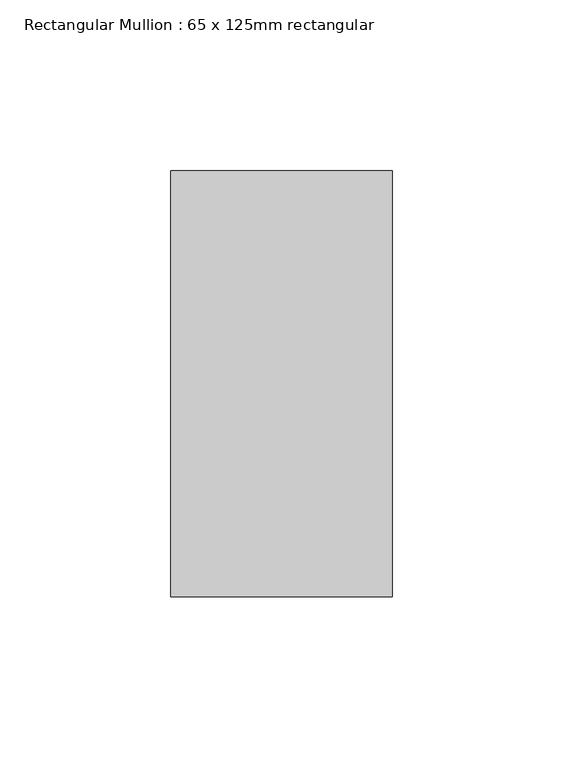
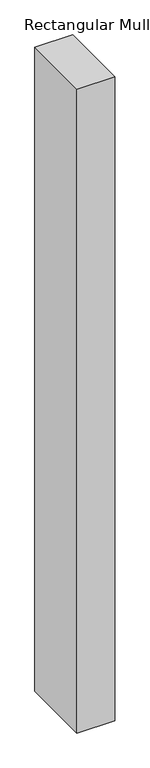
"""IFC4 building model written with IfcOpenShell, lengths in millimetres: member geometry, Rectangular Mullion : 65 x 125mm rectangular."""

from ifc_helpers import new_model, si_unit, frame, origin, place, context, project, spatial, polyline, outline, extrude, source, transform, mapped, element, save


def rectangular_mullion_65_x_125mm_rectangular_013ac084(model_context):
    return source(origin(), model_context, "Body", "SweptSolid", [
        extrude(outline(polyline([(0.0, 62.5), (0.0, -62.5), (-65.0, -62.5), (-65.0, 62.5), (0.0, 62.5)])), frame((0.0, 0.0, -1170.0), z_axis=(0.0, 0.0, 1.0), x_axis=(1.0, 0.0, 0.0)), (0.0, 0.0, 1.0), 1170.0),
    ])


if __name__ == "__main__":
    model = new_model("IFC4")
    model_context = context("Model", 3, world=origin())
    ifc_project = project(units=[si_unit("LENGTHUNIT", "METRE", prefix="MILLI")], contexts=[model_context])
    site = spatial("IfcSite", under=ifc_project)
    building = spatial("IfcBuilding", under=site)
    placement = place(None, origin())
    rectangular_mullion_65_x_125mm_rectangular_shape = rectangular_mullion_65_x_125mm_rectangular_013ac084(model_context)
    element("IfcMember", 1, ObjectType="Rectangular Mullion : 65 x 125mm rectangular", at=placement, inside=building, context=model_context, shape_type="MappedRepresentation", body=[
        mapped(rectangular_mullion_65_x_125mm_rectangular_shape, transform((0.0, 0.0, 0.0), x_axis=(1.0, 0.0, 0.0), y_axis=(0.0, 1.0, 0.0), z_axis=(0.0, 0.0, 1.0))),
    ])
    save(model, "model.ifc")

# Revit data of these elements
# Type "Rectangular Mullion : 65 x 125mm rectangular"
#   built-in parameter 1007304 = 0.410105 (stored number, unit not read)
#   built-in parameter 1007301 = 0.106627 (stored number, unit not read)
#   built-in parameter 1007300 = 0.106627 (stored number, unit not read)
# Element 1 (IfcMember, "Rectangular Mullion : 65 x 125mm rectangular")
#   Materials on its faces: "Aluminum"
# Materials
#   "Aluminum": class "Metal", colour RGB 244 245 246, transparency 0, Description = "Aluminum 6061", Cost = 0
